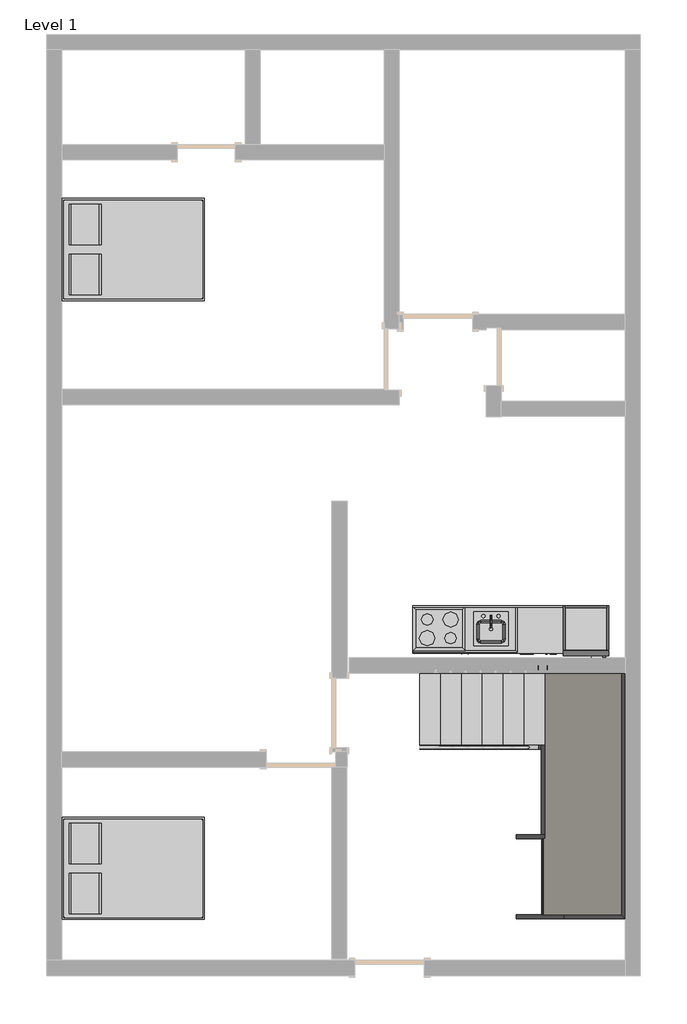
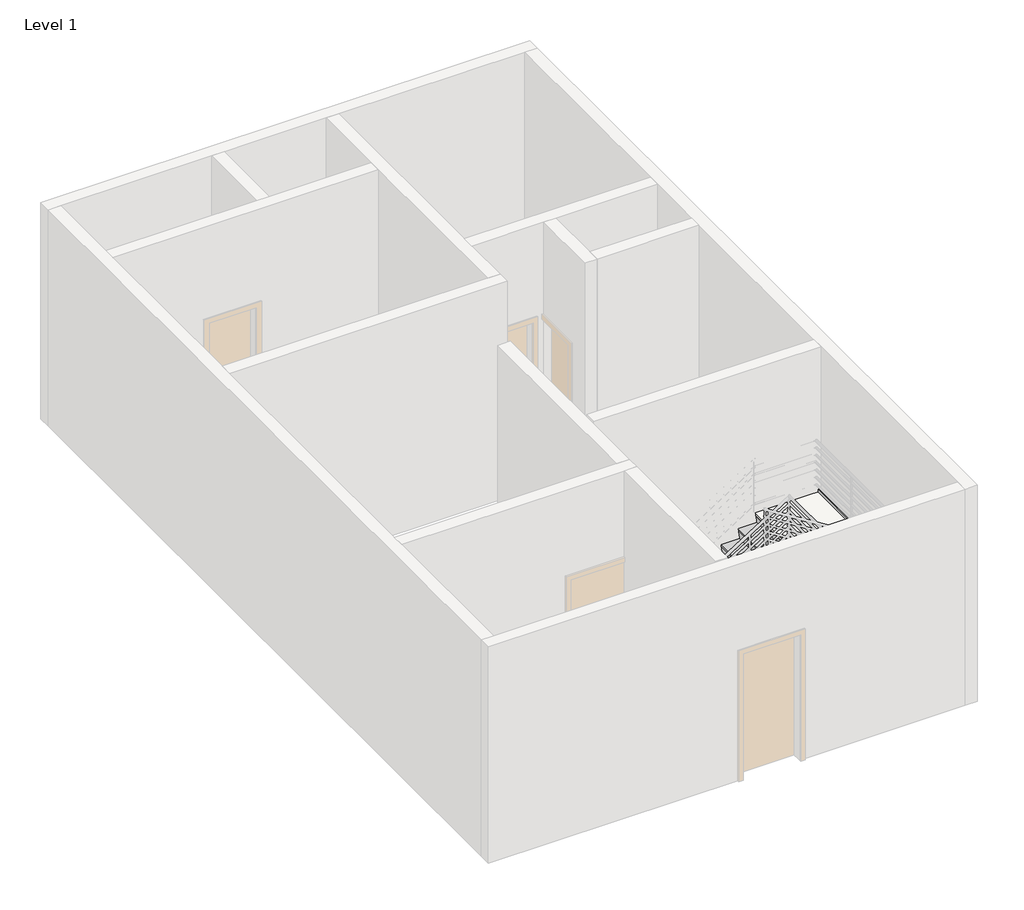
# One storey, part 4 of 4: 8 members, 4 proxies, 3 furniture elements, 2 stair flights, 1 flow terminal, 1 slab.
"""IFC4 building model written with IfcOpenShell, lengths in millimetres."""

from ifc_helpers import new_model, si_unit, frame, origin, place, context, project, spatial, polyline, outline, extrude, faceted_brep, transform, mapped, element, save
from components import m_cook_top_4_unit2_0615_x_500mm_249f3515, m_dishwasher_610_x_610_x_875mm_54ecfc4c, m_kitchenette_medium_1372mm_e05c6bec, m_refrigerator_600_x_660mm_a466bf94, m_sink_kitchen_island_450_x_450mm_f969cf2d, m_bed_box_1346_x_1880mm_double_b32eb57e, m_counter_top_w_sink_hole_600mm_depth_0a237b63, non_monolithic_landing_cc3d4867, stair_flight_50mm_tread_25mm_nosing_13mm_riser_f0f518ff, stair_flight_50mm_tread_25mm_nosing_13mm_riser_dbe7f446

model = new_model("IFC4")

# Units and contexts
model_context = context("Model", 3, world=origin())
ifc_project = project(units=[si_unit("LENGTHUNIT", "METRE", prefix="MILLI")], contexts=[model_context])

# Site, building, storey
site = spatial("IfcSite", under=ifc_project)
building = spatial("IfcBuilding", under=site)
storey = spatial("IfcBuildingStorey", under=building, Name="Level 1", Elevation=0.0)

# Proxies
placement = place(None, origin())
m_cook_top_4_unit2_0615_x_500mm_shape = m_cook_top_4_unit2_0615_x_500mm_249f3515(model_context)
element("IfcBuildingElementProxy", 1, Name="M_Cook Top-4 Unit2 : 0615 x 500mm", ObjectType="M_Cook Top-4 Unit2 : 0615 x 500mm", at=placement, inside=storey, context=model_context, shape_type="MappedRepresentation", body=[
    mapped(m_cook_top_4_unit2_0615_x_500mm_shape, transform((-8488.6689427, 2695.7602653, 0.0), x_axis=(1.0, 0.0, 0.0), y_axis=(0.0, 1.0, 0.0), z_axis=(0.0, 0.0, 1.0))),
])
m_dishwasher_610_x_610_x_875mm_shape = m_dishwasher_610_x_610_x_875mm_54ecfc4c(model_context)
element("IfcBuildingElementProxy", 2, Name="M_Dishwasher : 610 x 610 x 875mm", ObjectType="M_Dishwasher : 610 x 610 x 875mm", at=placement, inside=storey, context=model_context, shape_type="MappedRepresentation", body=[
    mapped(m_dishwasher_610_x_610_x_875mm_shape, transform((-7539.1864112, 2429.1107005, 0.0), x_axis=(1.0, 0.0, 0.0), y_axis=(0.0, 1.0, 0.0), z_axis=(0.0, 0.0, 1.0))),
])
m_kitchenette_medium_1372mm_shape = m_kitchenette_medium_1372mm_e05c6bec(model_context)
element("IfcBuildingElementProxy", 3, Name="M_Kitchenette - Medium : 1372mm", ObjectType="M_Kitchenette - Medium : 1372mm", at=placement, inside=storey, context=model_context, shape_type="MappedRepresentation", body=[
    mapped(m_kitchenette_medium_1372mm_shape, transform((-8164.4066477, 3000.7602653, 0.0), x_axis=(1.0, 0.0, 0.0), y_axis=(0.0, 1.0, 0.0), z_axis=(0.0, 0.0, 1.0))),
])
m_refrigerator_600_x_660mm_shape = m_refrigerator_600_x_660mm_a466bf94(model_context)
element("IfcBuildingElementProxy", 4, Name="M_Refrigerator : 600 x 660mm", ObjectType="M_Refrigerator : 600 x 660mm", at=placement, inside=storey, context=model_context, shape_type="MappedRepresentation", body=[
    mapped(m_refrigerator_600_x_660mm_shape, transform((-6497.8678001, 2704.5451751, 0.0), x_axis=(1.0, 0.0, 0.0), y_axis=(0.0, 1.0, 0.0), z_axis=(0.0, 0.0, 1.0))),
])

# Flow terminal
m_sink_kitchen_island_450_x_450mm_shape = m_sink_kitchen_island_450_x_450mm_f969cf2d(model_context)
element("IfcFlowTerminal", 5, ObjectType="M_Sink Kitchen-Island : 450 x 450mm", at=placement, inside=storey, context=model_context, shape_type="MappedRepresentation", body=[
    mapped(m_sink_kitchen_island_450_x_450mm_shape, transform((-7818.3581833, 2693.4148642, 0.0), x_axis=(1.0, 0.0, 0.0), y_axis=(0.0, 1.0, 0.0), z_axis=(0.0, 0.0, 1.0))),
])

# Furniture
m_bed_box_1346_x_1880mm_double_shape = m_bed_box_1346_x_1880mm_double_b32eb57e(model_context)
element("IfcFurniture", 6, ObjectType="M_Bed-Box : 1346 x 1880mm - Double", at=placement, inside=storey, context=model_context, shape_type="MappedRepresentation", body=[
    mapped(m_bed_box_1346_x_1880mm_double_shape, transform((-12750.0984509, 7352.4078063, 0.0), x_axis=(0.0, 1.0000000000000002, 0.0), y_axis=(-1.0000000000000002, 0.0, 0.0), z_axis=(0.0, 0.0, 1.0))),
])
element("IfcFurniture", 7, ObjectType="M_Bed-Box : 1346 x 1880mm - Double", at=placement, inside=storey, context=model_context, shape_type="MappedRepresentation", body=[
    mapped(m_bed_box_1346_x_1880mm_double_shape, transform((-12750.0984509, -797.7921937, 0.0), x_axis=(0.0, 0.9999999999999999, 0.0), y_axis=(-0.9999999999999999, 0.0, 0.0), z_axis=(0.0, 0.0, 1.0))),
])
m_counter_top_w_sink_hole_600mm_depth_shape = m_counter_top_w_sink_hole_600mm_depth_0a237b63(model_context)
element("IfcFurniture", 8, ObjectType="M_Counter Top w Sink Hole : 600mm Depth", at=placement, inside=storey, context=model_context, shape_type="MappedRepresentation", body=[
    mapped(m_counter_top_w_sink_hole_600mm_depth_shape, transform((-7631.2066477, 3000.7602653, 0.0), x_axis=(1.0, 0.0, 0.0), y_axis=(0.0, 1.0, 0.0), z_axis=(0.0, 0.0, 1.0))),
])

# Members
element("IfcMember", 9, ObjectType="Stringer - 50mm Width", at=placement, inside=storey, context=model_context, shape_type="SweptSolid", body=[
    extrude(outline(polyline([(215.089535, -8739.5726707), (0.0, -8739.5726707), (0.0, -8331.3139379), (864.7850313, -6963.8726072), (1264.7850313, -7079.7416672), (215.089535, -8739.5726707)])), frame((0.0, 2160.3311514, 0.0), z_axis=(0.0, 1.0, 0.0), x_axis=(0.0, 0.0, 1.0)), (0.0, 0.0, 1.0), 50.0),
])
element("IfcMember", 10, ObjectType="Stringer - 50mm Width", at=placement, inside=storey, context=model_context, shape_type="SweptSolid", body=[
    extrude(outline(polyline([(215.089535, -8739.5726707), (0.0, -8739.5726707), (0.0, -8331.3139379), (753.6703666, -7139.5726707), (1226.9472425, -7139.5726707), (215.089535, -8739.5726707)])), frame((0.0, 1110.3053702, 0.0), z_axis=(0.0, 1.0, 0.0), x_axis=(0.0, 0.0, 1.0)), (0.0, 0.0, 1.0), 50.0),
])
element("IfcMember", 11, ObjectType="Stringer - 50mm Width", at=placement, inside=storey, context=model_context, shape_type="SweptSolid", body=[
    extrude(outline(polyline([(864.7850313, -6940.2727343), (1264.7850313, -6824.4036743), (2128.1330133, -8189.5726707), (1654.8561374, -8189.5726707), (864.7850313, -6940.2727343)])), frame((0.0, -1119.1062768, 0.0), z_axis=(0.0, 1.0, 0.0), x_axis=(0.0, 0.0, 1.0)), (0.0, 0.0, 1.0), 50.0),
])
element("IfcMember", 12, ObjectType="Stringer - 50mm Width", at=placement, inside=storey, context=model_context, shape_type="SweptSolid", body=[
    extrude(outline(polyline([(959.2039634, -7089.5726707), (1432.4808393, -7089.5726707), (2128.1330133, -8189.5726707), (1654.8561374, -8189.5726707), (959.2039634, -7089.5726707)])), frame((0.0, -69.0804955, 0.0), z_axis=(0.0, 1.0, 0.0), x_axis=(0.0, 0.0, 1.0)), (0.0, 0.0, 1.0), 50.0),
])
element("IfcMember", 13, ObjectType="Stringer - 50mm Width", at=placement, inside=storey, context=model_context, shape_type="Brep", body=[
    faceted_brep([(-6824.4036743, -1069.1062768, 1264.7850313), (-6824.4036743, -1119.1062768, 1264.7850313), (-6039.5468895, -1119.1062768, 1264.7850313), (-6089.5468895, -1069.1062768, 1264.7850313), (-6940.2727343, -1069.1062768, 864.7850313), (-6089.5468895, -1069.1062768, 864.7850313), (-6940.2727343, -1119.1062768, 864.7850313), (-6039.5468895, -1119.1062768, 864.7850313)], [[[0, 1, 2, 3]], [[4, 0, 3, 5]], [[6, 4, 5, 7]], [[1, 6, 7, 2]], [[1, 0, 4, 6]], [[2, 7, 5, 3]]]),
])
element("IfcMember", 14, ObjectType="Stringer - 50mm Width", at=placement, inside=storey, context=model_context, shape_type="SweptSolid", body=[
    extrude(outline(polyline([(-6039.5468895, -1119.1062768), (-6089.5468895, -1069.1062768), (-6089.5468895, 2160.3311514), (-6039.5468895, 2210.3311514), (-6039.5468895, -1119.1062768)])), frame((0.0, 0.0, 864.7850313), z_axis=(0.0, 0.0, 1.0), x_axis=(1.0, 0.0, 0.0)), (0.0, 0.0, 1.0), 400.0),
])
element("IfcMember", 15, ObjectType="Stringer - 50mm Width", at=placement, inside=storey, context=model_context, shape_type="Brep", body=[
    faceted_brep([(-6089.5468895, 2160.3311514, 1264.7850313), (-6039.5468895, 2210.3311514, 1264.7850313), (-7079.7416672, 2210.3311514, 1264.7850313), (-7079.7416672, 2160.3311514, 1264.7850313), (-6089.5468895, 2160.3311514, 864.7850313), (-6963.8726072, 2160.3311514, 864.7850313), (-6039.5468895, 2210.3311514, 864.7850313), (-6963.8726072, 2210.3311514, 864.7850313)], [[[0, 1, 2, 3]], [[4, 0, 3, 5]], [[6, 4, 5, 7]], [[1, 6, 7, 2]], [[1, 0, 4, 6]], [[2, 7, 5, 3]]]),
])
element("IfcMember", 16, ObjectType="Stringer - 50mm Width", at=placement, inside=storey, context=model_context, shape_type="SweptSolid", body=[
    extrude(outline(polyline([(-7139.5726707, 1160.3053702), (-7089.5726707, 1160.3053702), (-7089.5726707, -19.0804955), (-7139.5726707, -19.0804955), (-7139.5726707, 1160.3053702)])), frame((0.0, 0.0, 864.7850313), z_axis=(0.0, 0.0, 1.0), x_axis=(1.0, 0.0, 0.0)), (0.0, 0.0, 1.0), 400.0),
])

# Slab
non_monolithic_landing_shape = non_monolithic_landing_cc3d4867(model_context)
element("IfcSlab", 17, ObjectType="Non-Monolithic Landing", at=placement, inside=storey, context=model_context, shape_type="MappedRepresentation", body=[
    mapped(non_monolithic_landing_shape, transform((0.0, 0.0, 0.0), x_axis=(1.0, 0.0, 0.0), y_axis=(0.0, 1.0, 0.0), z_axis=(0.0, 0.0, 1.0))),
])

# Stair flights
stair_flight_50mm_tread_25mm_nosing_13mm_riser_shape = stair_flight_50mm_tread_25mm_nosing_13mm_riser_f0f518ff(model_context)
element("IfcStairFlight", 18, ObjectType="50mm Tread 25mm Nosing 13mm Riser", at=placement, inside=storey, context=model_context, shape_type="MappedRepresentation", body=[
    mapped(stair_flight_50mm_tread_25mm_nosing_13mm_riser_shape, transform((0.0, 0.0, 0.0), x_axis=(1.0, 0.0, 0.0), y_axis=(0.0, 1.0, 0.0), z_axis=(0.0, 0.0, 1.0))),
])
stair_flight_50mm_tread_25mm_nosing_13mm_riser_2_shape = stair_flight_50mm_tread_25mm_nosing_13mm_riser_dbe7f446(model_context)
element("IfcStairFlight", 19, ObjectType="50mm Tread 25mm Nosing 13mm Riser", at=placement, inside=storey, context=model_context, shape_type="MappedRepresentation", body=[
    mapped(stair_flight_50mm_tread_25mm_nosing_13mm_riser_2_shape, transform((0.0, 0.0, 0.0), x_axis=(1.0, 0.0, 0.0), y_axis=(0.0, 1.0, 0.0), z_axis=(0.0, 0.0, 1.0))),
])

save(model, "model.ifc")

# Revit data of these elements
# Type "M_Cook Top-4 Unit2 : 0615 x 500mm"
#   Depth = 500 mm
#   Width = 615 mm
#   Burner Material = Steel, Chrome Plated
#   Cooktop Material = Steel, Polished
#   Default Elevation = 0
#   Assembly Code = ""
# Type "M_Dishwasher : 610 x 610 x 875mm"
#   Label = "DW"
#   Depth = 610 mm
#   Height = 875 mm
#   Width = 610 mm
#   Dishwasher Material = Steel, Paint Finish, Ivory, Glossy
#   Panel Face Material = Plastic, Opaque Black
#   Default Elevation = 0
# Type "M_Kitchenette - Medium : 1372mm"
#   Counter Length = 1980 mm
#   Cabinet Width = 1372 mm
#   Cabinet Height = 900 mm
#   Cabinet Depth = 610 mm
#   Toe Depth = 35 mm
#   Toe Height = 100 mm
#   Cabinet Material = Cabinets
#   Door/Drawer Material = Cabinets
#   Handle Material = Cabinets - Handles
#   Default Elevation = 0
# Type "M_Refrigerator : 600 x 660mm"
#   Label = "REF."
#   Depth = 660 mm
#   Height = 1830 mm
#   Width = 600 mm
#   Material = Steel, Paint Finish, Ivory, Matte
#   Description = (empty or 0)
#   Default Elevation = 0
# Type "M_Sink Kitchen-Island : 450 x 450mm"
#   Counter Height [instance default] = 900 mm
#   Depth = 450 mm
#   Width = 450 mm
#   Fixture Material = Steel, Polished
#   Sink Material = Steel, Polished
#   Default Elevation = 0
# Type "M_Bed-Box : 1346 x 1880mm - Double"
#   Length = 1880 mm
#   Width = 1346 mm
#   Frame Material = Birch
#   Mattress Material = Linen, White
#   Default Elevation = 0
# Type "M_Counter Top w Sink Hole : 600mm Depth"
#   Counter Thickness = 40 mm
#   Depth = 625 mm
#   Height = 900 mm
#   Length [instance default] = 2500 mm
#   Sink Location [instance default] = 1200 mm
#   Sink Location To Wall [instance default] = 100 mm
#   Sink Opening Depth [instance default] = 378 mm
#   Sink Opening Width [instance default] = 587 mm
#   Counter Top Material = none
#   Default Elevation = 0
# Element 1 (IfcBuildingElementProxy, "M_Cook Top-4 Unit2 : 0615 x 500mm")
#   Phase Created = New Construction
#   Materials on its faces: "Steel, Polished", "Steel, Chrome Plated"
# Element 2 (IfcBuildingElementProxy, "M_Dishwasher : 610 x 610 x 875mm")
#   Phase Created = New Construction
#   Materials on its faces: "Steel, Paint Finish, Ivory, Glossy", "Plastic, Opaque Black"
# Element 3 (IfcBuildingElementProxy, "M_Kitchenette - Medium : 1372mm")
#   Phase Created = New Construction
#   Materials on its faces: "Cabinets", "Cabinets - Handles"
# Element 4 (IfcBuildingElementProxy, "M_Refrigerator : 600 x 660mm")
#   Phase Created = New Construction
#   Materials on its faces: "Steel, Paint Finish, Ivory, Matte", "Steel, Chrome Plated"
# Element 5 (IfcFlowTerminal, "M_Sink Kitchen-Island : 450 x 450mm")
#   Mark = "1"
#   Counter Height = 900 mm
#   Phase Created = New Construction
#   Materials on its faces: "Steel, Polished"
# Elements 6, 7 (IfcFurniture, "M_Bed-Box : 1346 x 1880mm - Double")
#   Phase Created = New Construction
#   Materials on its faces: "Birch", "Linen, White"
# Element 8 (IfcFurniture, "M_Counter Top w Sink Hole : 600mm Depth")
#   Sink Opening Width = 400 mm
#   Sink Opening Depth = 350 mm
#   Sink Location To Wall = 160 mm
#   Sink Location = 1025 mm
#   Length = 1980 mm
#   Phase Created = New Construction
#   Materials on its faces: "Counter Top"
# Elements 9, 10, 11, 12, 13, 14, 15, 16 (IfcMember, "Stringer - 50mm Width")
#   Phase Created = New Construction
# Element 17 (IfcSlab, "Non-Monolithic Landing")
#   Phase Created = New Construction
# Elements 18, 19 (IfcStairFlight, "50mm Tread 25mm Nosing 13mm Riser")
#   Phase Created = New Construction
# Materials
#   "Steel, Chrome Plated": class "Metal", colour RGB 244 244 244, transparency 0, Description = "Chromiuim plated steel", Cost = 0
#   "Steel, Polished": class "Metal", colour RGB 57 57 57, transparency 0, Description = "Polished steel", Cost = 0
#   "Steel, Paint Finish, Ivory, Glossy": class "Metal", colour RGB 247 247 239, transparency 0, Description = "Steel, paint finish, ivory, glossy", Cost = 0
#   "Plastic, Opaque Black": class "Plastic", colour RGB 0 0 0, transparency 0.7, Description = "Plastic, generic, opaque black", Cost = 0
#   "Cabinets": colour RGB 249 249 249, transparency 0
#   "Cabinets - Handles": class "Metal", colour RGB 57 57 57, transparency 0
#   "Steel, Paint Finish, Ivory, Matte": class "Metal", colour RGB 247 247 239, transparency 0, Description = "Steel, paint finish, ivory, matte", Cost = 0
#   "Birch": class "Wood", colour RGB 224 178 126, transparency 0, Description = "Betula Alleghaniensis", Cost = 0
#   "Linen, White": class "Textile", colour RGB 247 247 239, transparency 0, Description = "Linen, white", Cost = 0
#   "Counter Top": class "Wood", colour RGB 226 177 128, transparency 0
